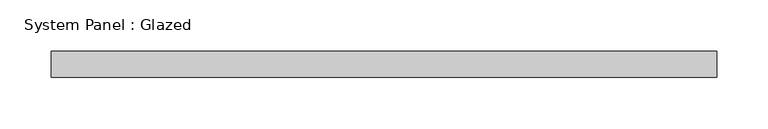
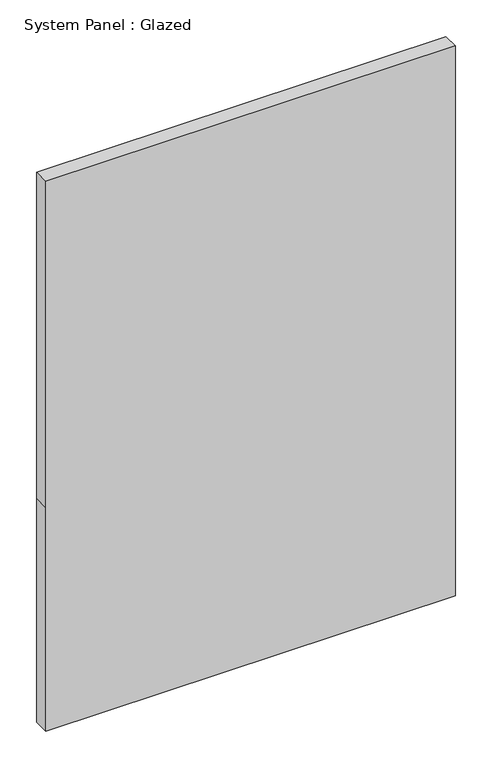
"""IFC4 building model written with IfcOpenShell, lengths in millimetres: plate geometry, System Panel : Glazed."""

from ifc_helpers import new_model, si_unit, frame, origin, place, context, project, spatial, polyline, outline, extrude, source, transform, mapped, element, save


def system_panel_glazed_d3cf7d22(model_context):
    return source(origin(), model_context, "Body", "SweptSolid", [
        extrude(outline(polyline([(0.0, -323.85), (0.0, 323.85), (373.9836648, 323.85), (919.084162, 323.85), (919.084162, -323.85), (373.9836648, -323.85), (0.0, -323.85)])), frame((0.0, 19.05, 0.0), z_axis=(0.0, 1.0, 0.0), x_axis=(0.0, 0.0, 1.0)), (0.0, 0.0, 1.0), 25.4),
    ])


if __name__ == "__main__":
    model = new_model("IFC4")
    model_context = context("Model", 3, world=origin())
    ifc_project = project(units=[si_unit("LENGTHUNIT", "METRE", prefix="MILLI")], contexts=[model_context])
    site = spatial("IfcSite", under=ifc_project)
    building = spatial("IfcBuilding", under=site)
    placement = place(None, origin())
    system_panel_glazed_shape = system_panel_glazed_d3cf7d22(model_context)
    element("IfcPlate", 1, ObjectType="System Panel : Glazed", at=placement, inside=building, context=model_context, shape_type="MappedRepresentation", body=[
        mapped(system_panel_glazed_shape, transform((0.0, 0.0, 0.0), x_axis=(1.0, 0.0, 0.0), y_axis=(0.0, 1.0, 0.0), z_axis=(0.0, 0.0, 1.0))),
    ])
    save(model, "model.ifc")

# Revit data of these elements
# Type "System Panel : Glazed"
#   Construction Type Id = "GSP4R"
#   Analytic Construction = "1/8 in Pilkington single glazing"
#   Visual Light Transmittance = 0.9
#   Solar Heat Gain Coefficient = 0.86
#   Heat Transfer Coefficient (U) = 1.18115 BTU/(h·ft²·°F)
#   Define Thermal Properties by = 1
# Element 1 (IfcPlate, "System Panel : Glazed")
#   Materials on its faces: "Glass"
# Materials
#   "Glass": class "Glass", colour RGB 0 128 192, transparency 0.75, Description = "Soda Lime Glass", Cost = 0
